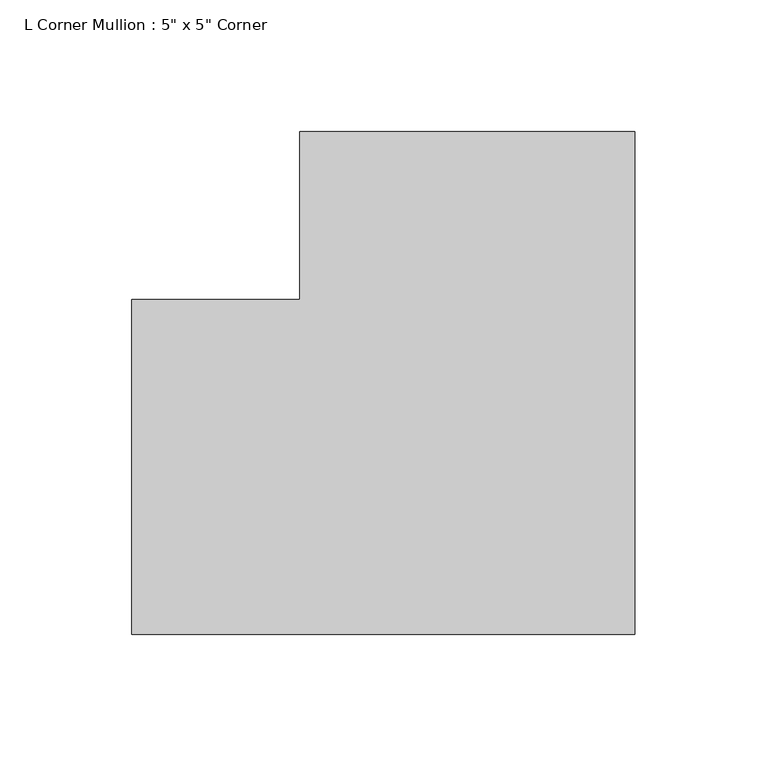
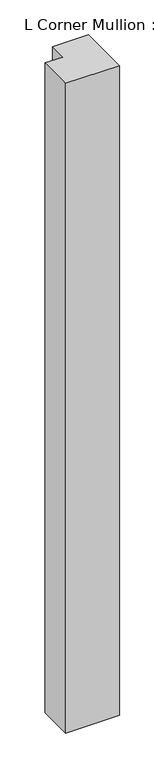
"""IFC4 building model written with IfcOpenShell, lengths in millimetres: member geometry."""

from ifc_helpers import new_model, si_unit, frame, origin, place, context, project, spatial, polyline, outline, extrude, source, transform, mapped, element, save


def member_cc254986(model_context):
    return source(origin(), model_context, "Body", "SweptSolid", [
        extrude(outline(polyline([(63.5, 127.0), (63.5, -63.5), (-127.0, -63.5), (-127.0, 63.5), (-63.5, 63.5), (-63.5, 127.0), (63.5, 127.0)])), frame((0.0, 0.0, -2438.4), z_axis=(0.0, 0.0, 1.0), x_axis=(1.0, 0.0, 0.0)), (0.0, 0.0, 1.0), 2438.4),
    ])


if __name__ == "__main__":
    model = new_model("IFC4")
    model_context = context("Model", 3, world=origin())
    ifc_project = project(units=[si_unit("LENGTHUNIT", "METRE", prefix="MILLI")], contexts=[model_context])
    site = spatial("IfcSite", under=ifc_project)
    building = spatial("IfcBuilding", under=site)
    placement = place(None, origin())
    member_shape = member_cc254986(model_context)
    element("IfcMember", 1, ObjectType="L Corner Mullion : 5\" x 5\" Corner", at=placement, inside=building, context=model_context, shape_type="MappedRepresentation", body=[
        mapped(member_shape, transform((0.0, 0.0, 0.0), x_axis=(1.0, 0.0, 0.0), y_axis=(0.0, 1.0, 0.0), z_axis=(0.0, 0.0, 1.0))),
    ])
    save(model, "model.ifc")

# Revit data of these elements
# Type "L Corner Mullion : 5\" x 5\" Corner"
#   built-in parameter 1007355 = 0.416667 (stored number, unit not read)
#   built-in parameter 1007354 = 0.416667 (stored number, unit not read)
#   built-in parameter 1007304 = 0.416667 (stored number, unit not read)
# Element 1 (IfcMember, "L Corner Mullion : 5\" x 5\" Corner")
#   Materials on its faces: "mullions"
# Materials
#   "mullions": class "Generic", colour RGB 120 120 120, transparency 0, Cost = 0
